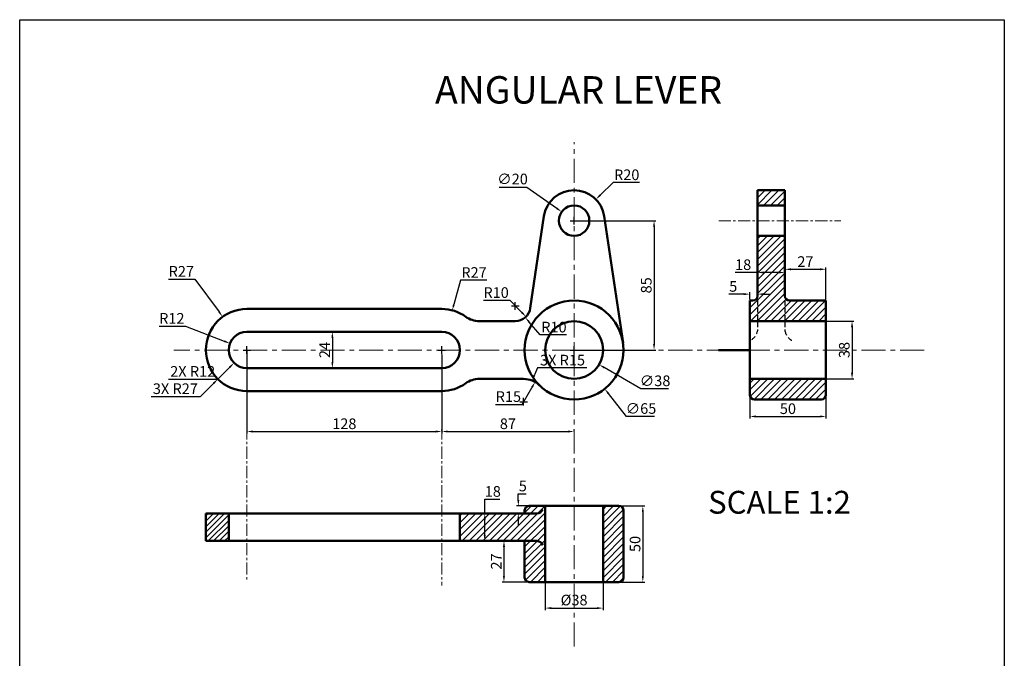
# Model space of a CAD drawing. Units: millimetres. Extents: x 161 to 808, y -21 to 750.
# Tile 2 of 2: x 161 to 808, y 330 to 750. Entities that reach past the tile are written whole.
import ezdxf

# ---------------------------------------------------------------- set-up
doc = ezdxf.new("R2010")
doc.units = ezdxf.units.MM
doc.header["$LTSCALE"] = 0.5
doc.linetypes.add('CENTER', pattern=[50.8, 31.75, -6.35, 6.35, -6.35])
doc.linetypes.add('DASHED', pattern=[19.05, 12.7, -6.35])
for name, color, linetype, lineweight in [('M-CNTR', 1, 'CENTER', 18), ('M-DIMS', 2, 'Continuous', 25), ('M-HATC', 8, 'Continuous', 18), ('M-HIDN', 6, 'DASHED', 25), ('M-OUTL', 7, 'Continuous', 50), ('M-TEXT', 3, 'Continuous', 25), ('M-TTLB', 7, 'Continuous', 25)]:
    doc.layers.add(name, color=color, linetype=linetype, lineweight=lineweight)
doc.styles.get("Standard").update_dxf_attribs({"font": 'arial.ttf'})
doc.dimstyles.new('ISO-25', dxfattribs={"dimtxt": 7, "dimasz": 4, "dimexe": 1.25, "dimexo": 0.625, "dimtad": 1, "dimtoh": 1, "dimtxsty": 'Standard', "dimcen": 2.5, "dimadec": 0, "dimazin": 0, "dimtfac": 1, "dimtofl": 0, "dimtmove": 0, "dimatfit": 3, "dimfxl": 1, "dimarcsym": 0})

# ---------------------------------------------------------------- blocks, each defined once
blk = doc.blocks.new('*D1')
at = {"layer": 'Defpoints', "color": 0, "ltscale": 0.5, "transparency": 16777216}
for p in [(294.56, 554.39), (310.51, 532.61)]:
    blk.add_point(p, dxfattribs=at)
at = {"layer": 'M-DIMS', "color": 0, "lineweight": -2, "ltscale": 0.5, "transparency": 16777216}
for p, q in [((258.99, 579.26), (276.35, 579.26)), ((276.35, 579.26), (292.2, 557.62)), ((308.01, 532.61), (313.01, 532.61)), ((310.51, 530.11), (310.51, 535.11))]:
    blk.add_line(p, q, dxfattribs=at)
at = {"layer": 'M-DIMS', "color": 0, "ltscale": 0.5, "transparency": 16777216}
blk.add_solid([(292.73, 558.01), (291.66, 557.23), (294.56, 554.39)], dxfattribs=at)
at = {"layer": 'M-DIMS', "color": 0, "ltscale": 0.5, "transparency": 16777216, "insert": (267.36, 583.4), "char_height": 7, "attachment_point": 5}
blk.add_mtext('R27', dxfattribs=at)
blk = doc.blocks.new('*D2')
at = {"layer": 'Defpoints', "color": 0, "ltscale": 0.5, "transparency": 16777216}
for p in [(299.33, 536.97), (310.51, 532.61)]:
    blk.add_point(p, dxfattribs=at)
at = {"layer": 'M-DIMS', "color": 0, "lineweight": -2, "ltscale": 0.5, "transparency": 16777216}
for p, q in [((252.81, 548.36), (270.09, 548.36)), ((270.09, 548.36), (295.6, 538.42)), ((308.01, 532.61), (313.01, 532.61)), ((310.51, 530.11), (310.51, 535.11))]:
    blk.add_line(p, q, dxfattribs=at)
at = {"layer": 'M-DIMS', "color": 0, "ltscale": 0.5, "transparency": 16777216}
blk.add_solid([(295.85, 539.04), (295.36, 537.8), (299.33, 536.97)], dxfattribs=at)
at = {"layer": 'M-DIMS', "color": 0, "ltscale": 0.5, "transparency": 16777216, "insert": (261.14, 552.5), "char_height": 7, "attachment_point": 5}
blk.add_mtext('R12', dxfattribs=at)
blk = doc.blocks.new('*D3')
at = {"layer": 'Defpoints', "color": 0, "ltscale": 0.5, "transparency": 16777216}
for p in [(486.86, 561.61), (493.9, 554.51)]:
    blk.add_point(p, dxfattribs=at)
at = {"layer": 'M-DIMS', "color": 0, "lineweight": -2, "ltscale": 0.5, "transparency": 16777216}
for p, q in [((465.9, 565.26), (483.23, 565.26)), ((483.23, 565.26), (491.08, 557.35))]:
    blk.add_line(p, q, dxfattribs=at)
at = {"layer": 'M-DIMS', "color": 0, "ltscale": 0.5, "transparency": 16777216}
blk.add_solid([(491.56, 557.82), (490.61, 556.88), (493.9, 554.51)], dxfattribs=at)
at = {"layer": 'M-DIMS', "color": 0, "ltscale": 0.5, "transparency": 16777216, "insert": (474.25, 569.46), "char_height": 7, "attachment_point": 5}
blk.add_mtext('R10', dxfattribs=at)
blk = doc.blocks.new('*D4')
at = {"layer": 'Defpoints', "color": 0, "ltscale": 0.5, "transparency": 16777216}
for p in [(445.48, 558.69), (438.51, 532.61)]:
    blk.add_point(p, dxfattribs=at)
at = {"layer": 'M-DIMS', "color": 0, "lineweight": -2, "ltscale": 0.5, "transparency": 16777216}
for p, q in [((450.77, 578.5), (446.51, 562.56)), ((468.12, 578.5), (450.77, 578.5)), ((436.01, 532.61), (441.01, 532.61)), ((438.51, 530.11), (438.51, 535.11))]:
    blk.add_line(p, q, dxfattribs=at)
at = {"layer": 'M-DIMS', "color": 0, "ltscale": 0.5, "transparency": 16777216}
blk.add_solid([(445.87, 562.73), (447.16, 562.39), (445.48, 558.69)], dxfattribs=at)
at = {"layer": 'M-DIMS', "color": 0, "ltscale": 0.5, "transparency": 16777216, "insert": (459.76, 582.64), "char_height": 7, "attachment_point": 5}
blk.add_mtext('R27', dxfattribs=at)
blk = doc.blocks.new('*D5')
at = {"layer": 'Defpoints', "color": 0, "ltscale": 0.5, "transparency": 16777216}
for p in [(539.81, 631.6), (525.51, 617.61)]:
    blk.add_point(p, dxfattribs=at)
at = {"layer": 'M-DIMS', "color": 0, "lineweight": -2, "ltscale": 0.5, "transparency": 16777216}
for p, q in [((551.11, 642.66), (542.66, 634.4)), ((568.44, 642.66), (551.11, 642.66)), ((523.01, 617.61), (528.01, 617.61)), ((525.51, 615.11), (525.51, 620.11))]:
    blk.add_line(p, q, dxfattribs=at)
at = {"layer": 'M-DIMS', "color": 0, "ltscale": 0.5, "transparency": 16777216}
blk.add_solid([(542.2, 634.87), (543.13, 633.92), (539.81, 631.6)], dxfattribs=at)
at = {"layer": 'M-DIMS', "color": 0, "ltscale": 0.5, "transparency": 16777216, "insert": (560.09, 646.86), "char_height": 7, "attachment_point": 5}
blk.add_mtext('R20', dxfattribs=at)
blk = doc.blocks.new('*D6')
at = {"layer": 'Defpoints', "color": 0, "ltscale": 0.5, "transparency": 16777216}
for p in [(509.1, 542.18), (541.92, 523.03)]:
    blk.add_point(p, dxfattribs=at)
at = {"layer": 'M-DIMS', "color": 0, "lineweight": -2, "ltscale": 0.5, "transparency": 16777216}
for p, q in [((523.01, 532.61), (528.01, 532.61)), ((525.51, 530.11), (525.51, 535.11)), ((569.29, 507.07), (545.38, 521.02)), ((587.57, 507.07), (569.29, 507.07))]:
    blk.add_line(p, q, dxfattribs=at)
at = {"layer": 'M-DIMS', "color": 0, "ltscale": 0.5, "transparency": 16777216}
blk.add_solid([(545.71, 521.59), (545.04, 520.44), (541.92, 523.03)], dxfattribs=at)
at = {"layer": 'M-DIMS', "color": 0, "ltscale": 0.5, "transparency": 16777216, "insert": (578.74, 511.46), "char_height": 7, "attachment_point": 5}
blk.add_mtext('∅38', dxfattribs=at)
blk = doc.blocks.new('*D7')
at = {"layer": 'Defpoints', "color": 0, "ltscale": 0.5, "transparency": 16777216}
for p in [(505.4, 558.14), (545.63, 507.08)]:
    blk.add_point(p, dxfattribs=at)
at = {"layer": 'M-DIMS', "color": 0, "lineweight": -2, "ltscale": 0.5, "transparency": 16777216}
for p, q in [((523.01, 532.61), (528.01, 532.61)), ((525.51, 530.11), (525.51, 535.11)), ((559.99, 488.86), (548.1, 503.94)), ((578.31, 488.86), (559.99, 488.86))]:
    blk.add_line(p, q, dxfattribs=at)
at = {"layer": 'M-DIMS', "color": 0, "ltscale": 0.5, "transparency": 16777216}
blk.add_solid([(548.63, 504.35), (547.58, 503.53), (545.63, 507.08)], dxfattribs=at)
at = {"layer": 'M-DIMS', "color": 0, "ltscale": 0.5, "transparency": 16777216, "insert": (569.46, 493.25), "char_height": 7, "attachment_point": 5}
blk.add_mtext('∅65', dxfattribs=at)
blk = doc.blocks.new('*D8')
at = {"layer": 'Defpoints', "color": 0, "ltscale": 0.5, "transparency": 16777216}
for p in [(517.37, 623.41), (533.66, 611.81)]:
    blk.add_point(p, dxfattribs=at)
at = {"layer": 'M-DIMS', "color": 0, "lineweight": -2, "ltscale": 0.5, "transparency": 16777216}
for p, q in [((476.23, 639.71), (494.48, 639.71)), ((494.48, 639.71), (514.11, 625.73)), ((523.01, 617.61), (528.01, 617.61)), ((525.51, 615.11), (525.51, 620.11))]:
    blk.add_line(p, q, dxfattribs=at)
at = {"layer": 'M-DIMS', "color": 0, "ltscale": 0.5, "transparency": 16777216}
blk.add_solid([(514.49, 626.27), (513.72, 625.19), (517.37, 623.41)], dxfattribs=at)
at = {"layer": 'M-DIMS', "color": 0, "ltscale": 0.5, "transparency": 16777216, "insert": (485.04, 644.1), "char_height": 7, "attachment_point": 5}
blk.add_mtext('∅20', dxfattribs=at)
blk = doc.blocks.new('*D9')
at = {"layer": 'Defpoints', "color": 0, "ltscale": 0.5, "transparency": 16777216}
for p in [(373.17, 544.61), (366.64, 520.61), (374.51, 520.61)]:
    blk.add_point(p, dxfattribs=at)
at = {"layer": 'M-DIMS', "color": 0, "lineweight": -2, "ltscale": 0.5, "transparency": 16777216}
for p, q in [((372.54, 544.61), (365.39, 544.61)), ((366.64, 540.61), (366.64, 524.61)), ((373.89, 520.61), (365.39, 520.61))]:
    blk.add_line(p, q, dxfattribs=at)
at = {"layer": 'M-DIMS', "color": 0, "ltscale": 0.5, "transparency": 16777216}
for points in [[(365.97, 540.61), (367.3, 540.61), (366.64, 544.61)], [(365.97, 524.61), (367.3, 524.61), (366.64, 520.61)]]:
    blk.add_solid(points, dxfattribs=at)
at = {"layer": 'M-DIMS', "color": 0, "ltscale": 0.5, "transparency": 16777216, "insert": (362.5, 532.61), "char_height": 7, "attachment_point": 5, "rotation": 90}
blk.add_mtext('24', dxfattribs=at)
blk = doc.blocks.new('*D10')
at = {"layer": 'Defpoints', "color": 0, "ltscale": 0.5, "transparency": 16777216}
for p in [(310.51, 532.61), (438.51, 530.11), (438.51, 479.03)]:
    blk.add_point(p, dxfattribs=at)
at = {"layer": 'M-DIMS', "color": 0, "lineweight": -2, "ltscale": 0.5, "transparency": 16777216}
for p, q in [((310.51, 531.98), (310.51, 477.78)), ((438.51, 529.48), (438.51, 477.78)), ((314.51, 479.03), (434.51, 479.03))]:
    blk.add_line(p, q, dxfattribs=at)
at = {"layer": 'M-DIMS', "color": 0, "ltscale": 0.5, "transparency": 16777216}
for points in [[(314.51, 479.69), (314.51, 478.36), (310.51, 479.03)], [(434.51, 479.69), (434.51, 478.36), (438.51, 479.03)]]:
    blk.add_solid(points, dxfattribs=at)
at = {"layer": 'M-DIMS', "color": 0, "ltscale": 0.5, "transparency": 16777216, "insert": (374.51, 483.22), "char_height": 7, "attachment_point": 5}
blk.add_mtext('128', dxfattribs=at)
blk = doc.blocks.new('*D11')
at = {"layer": 'Defpoints', "color": 0, "ltscale": 0.5, "transparency": 16777216}
for p in [(525.51, 617.61), (525.51, 532.61), (578.05, 532.61)]:
    blk.add_point(p, dxfattribs=at)
at = {"layer": 'M-DIMS', "color": 0, "lineweight": -2, "ltscale": 0.5, "transparency": 16777216}
for p, q in [((526.14, 617.61), (579.3, 617.61)), ((578.05, 613.61), (578.05, 536.61)), ((526.14, 532.61), (579.3, 532.61))]:
    blk.add_line(p, q, dxfattribs=at)
at = {"layer": 'M-DIMS', "color": 0, "ltscale": 0.5, "transparency": 16777216}
for points in [[(577.39, 613.61), (578.72, 613.61), (578.05, 617.61)], [(577.39, 536.61), (578.72, 536.61), (578.05, 532.61)]]:
    blk.add_solid(points, dxfattribs=at)
at = {"layer": 'M-DIMS', "color": 0, "ltscale": 0.5, "transparency": 16777216, "insert": (573.85, 575.11), "char_height": 7, "attachment_point": 5, "rotation": 90}
blk.add_mtext('85', dxfattribs=at)
blk = doc.blocks.new('*D12')
at = {"layer": 'Defpoints', "color": 0, "ltscale": 0.5, "transparency": 16777216}
for p in [(438.51, 479.03), (525.51, 479.03), (525.51, 479.03)]:
    blk.add_point(p, dxfattribs=at)
at = {"layer": 'M-DIMS', "color": 0, "lineweight": -2, "ltscale": 0.5, "transparency": 16777216}
for p, q in [((438.51, 479.65), (438.51, 480.28)), ((442.51, 479.03), (521.51, 479.03)), ((525.51, 479.65), (525.51, 480.28))]:
    blk.add_line(p, q, dxfattribs=at)
at = {"layer": 'M-DIMS', "color": 0, "ltscale": 0.5, "transparency": 16777216}
for points in [[(442.51, 479.69), (442.51, 478.36), (438.51, 479.03)], [(521.51, 479.69), (521.51, 478.36), (525.51, 479.03)]]:
    blk.add_solid(points, dxfattribs=at)
at = {"layer": 'M-DIMS', "color": 0, "ltscale": 0.5, "transparency": 16777216, "insert": (482.01, 483.22), "char_height": 7, "attachment_point": 5}
blk.add_mtext('87', dxfattribs=at)
blk = doc.blocks.new('*D13')
at = {"layer": 'Defpoints', "color": 0, "ltscale": 0.5, "transparency": 16777216}
for p in [(506.51, 380.12), (544.51, 380.12), (544.51, 362.97)]:
    blk.add_point(p, dxfattribs=at)
at = {"layer": 'M-DIMS', "color": 0, "lineweight": -2, "ltscale": 0.5, "transparency": 16777216}
for p, q in [((506.51, 379.49), (506.51, 361.72)), ((544.51, 379.49), (544.51, 361.72)), ((510.51, 362.97), (540.51, 362.97))]:
    blk.add_line(p, q, dxfattribs=at)
at = {"layer": 'M-DIMS', "color": 0, "ltscale": 0.5, "transparency": 16777216}
for points in [[(510.51, 363.64), (510.51, 362.31), (506.51, 362.97)], [(540.51, 363.64), (540.51, 362.31), (544.51, 362.97)]]:
    blk.add_solid(points, dxfattribs=at)
at = {"layer": 'M-DIMS', "color": 0, "ltscale": 0.5, "transparency": 16777216, "insert": (525.51, 367.37), "char_height": 7, "attachment_point": 5}
blk.add_mtext('%%C38', dxfattribs=at)
blk = doc.blocks.new('*D14')
at = {"layer": 'Defpoints', "color": 0, "ltscale": 0.5, "transparency": 16777216}
for p in [(496.01, 430.12), (488.86, 425.12), (496.01, 425.12)]:
    blk.add_point(p, dxfattribs=at)
at = {"layer": 'M-DIMS', "color": 0, "lineweight": -2, "ltscale": 0.5, "transparency": 16777216}
for p, q in [((488.86, 434.12), (488.86, 438.12)), ((488.86, 438.12), (494.12, 438.12)), ((495.39, 430.12), (487.61, 430.12)), ((495.39, 425.12), (487.61, 425.12)), ((488.86, 421.12), (488.86, 417.12))]:
    blk.add_line(p, q, dxfattribs=at)
at = {"layer": 'M-DIMS', "color": 0, "ltscale": 0.5, "transparency": 16777216}
for points in [[(488.19, 434.12), (489.53, 434.12), (488.86, 430.12)], [(488.19, 421.12), (489.53, 421.12), (488.86, 425.12)]]:
    blk.add_solid(points, dxfattribs=at)
at = {"layer": 'M-DIMS', "color": 0, "ltscale": 0.5, "transparency": 16777216, "insert": (491.8, 442.3), "char_height": 7, "attachment_point": 5}
blk.add_mtext('5', dxfattribs=at)
blk = doc.blocks.new('*D15')
at = {"layer": 'Defpoints', "color": 0, "ltscale": 0.5, "transparency": 16777216}
for p in [(479.65, 425.12), (466.78, 407.12), (479.65, 407.12)]:
    blk.add_point(p, dxfattribs=at)
at = {"layer": 'M-DIMS', "color": 0, "lineweight": -2, "ltscale": 0.5, "transparency": 16777216}
for p, q in [((466.78, 425.12), (466.78, 434.55)), ((466.78, 434.55), (476.79, 434.55)), ((479.03, 425.12), (465.53, 425.12)), ((466.78, 411.12), (466.78, 421.12)), ((479.03, 407.12), (465.53, 407.12))]:
    blk.add_line(p, q, dxfattribs=at)
at = {"layer": 'M-DIMS', "color": 0, "ltscale": 0.5, "transparency": 16777216}
for points in [[(466.11, 421.12), (467.45, 421.12), (466.78, 425.12)], [(466.11, 411.12), (467.45, 411.12), (466.78, 407.12)]]:
    blk.add_solid(points, dxfattribs=at)
at = {"layer": 'M-DIMS', "color": 0, "ltscale": 0.5, "transparency": 16777216, "insert": (472.1, 438.75), "char_height": 7, "attachment_point": 5}
blk.add_mtext('18', dxfattribs=at)
blk = doc.blocks.new('*D16')
at = {"layer": 'Defpoints', "color": 0, "ltscale": 0.5, "transparency": 16777216}
for p in [(691.04, 551.61), (691.04, 513.61), (708.18, 513.61)]:
    blk.add_point(p, dxfattribs=at)
at = {"layer": 'M-DIMS', "color": 0, "lineweight": -2, "ltscale": 0.5, "transparency": 16777216}
for p, q in [((691.66, 551.61), (709.43, 551.61)), ((708.18, 547.61), (708.18, 517.61)), ((691.66, 513.61), (709.43, 513.61))]:
    blk.add_line(p, q, dxfattribs=at)
at = {"layer": 'M-DIMS', "color": 0, "ltscale": 0.5, "transparency": 16777216}
for points in [[(707.52, 547.61), (708.85, 547.61), (708.18, 551.61)], [(707.52, 517.61), (708.85, 517.61), (708.18, 513.61)]]:
    blk.add_solid(points, dxfattribs=at)
at = {"layer": 'M-DIMS', "color": 0, "ltscale": 0.5, "transparency": 16777216, "insert": (703.98, 532.61), "char_height": 7, "attachment_point": 5, "rotation": 90}
blk.add_mtext('38', dxfattribs=at)
blk = doc.blocks.new('*D17')
at = {"layer": 'Defpoints', "color": 0, "ltscale": 0.5, "transparency": 16777216}
for p in [(641.04, 565.11), (646.04, 569.32), (646.04, 565.11)]:
    blk.add_point(p, dxfattribs=at)
at = {"layer": 'M-DIMS', "color": 0, "lineweight": -2, "ltscale": 0.5, "transparency": 16777216}
for p, q in [((641.04, 565.73), (641.04, 570.57)), ((646.04, 565.73), (646.04, 570.57)), ((637.04, 569.32), (627.15, 569.32)), ((650.04, 569.32), (654.04, 569.32))]:
    blk.add_line(p, q, dxfattribs=at)
at = {"layer": 'M-DIMS', "color": 0, "ltscale": 0.5, "transparency": 16777216}
for points in [[(637.04, 569.98), (637.04, 568.65), (641.04, 569.32)], [(650.04, 569.98), (650.04, 568.65), (646.04, 569.32)]]:
    blk.add_solid(points, dxfattribs=at)
at = {"layer": 'M-DIMS', "color": 0, "ltscale": 0.5, "transparency": 16777216, "insert": (630.09, 573.5), "char_height": 7, "attachment_point": 5}
blk.add_mtext('5', dxfattribs=at)
blk = doc.blocks.new('*D18')
at = {"layer": 'Defpoints', "color": 0, "ltscale": 0.5, "transparency": 16777216}
for p in [(664.04, 583.58), (646.04, 576.02), (664.04, 576.02)]:
    blk.add_point(p, dxfattribs=at)
at = {"layer": 'M-DIMS', "color": 0, "lineweight": -2, "ltscale": 0.5, "transparency": 16777216}
for p, q in [((646.04, 583.58), (631.29, 583.58)), ((646.04, 576.65), (646.04, 584.83)), ((660.04, 583.58), (650.04, 583.58)), ((664.04, 576.65), (664.04, 584.83))]:
    blk.add_line(p, q, dxfattribs=at)
at = {"layer": 'M-DIMS', "color": 0, "ltscale": 0.5, "transparency": 16777216}
for points in [[(650.04, 584.24), (650.04, 582.91), (646.04, 583.58)], [(660.04, 584.24), (660.04, 582.91), (664.04, 583.58)]]:
    blk.add_solid(points, dxfattribs=at)
at = {"layer": 'M-DIMS', "color": 0, "ltscale": 0.5, "transparency": 16777216, "insert": (636.61, 587.78), "char_height": 7, "attachment_point": 5}
blk.add_mtext('18', dxfattribs=at)
blk = doc.blocks.new('*D19')
at = {"layer": 'Defpoints', "color": 0, "ltscale": 0.5, "transparency": 16777216}
for p in [(691.04, 585.66), (664.04, 573.15), (691.04, 565.11)]:
    blk.add_point(p, dxfattribs=at)
at = {"layer": 'M-DIMS', "color": 0, "lineweight": -2, "ltscale": 0.5, "transparency": 16777216}
for p, q in [((664.04, 573.77), (664.04, 586.91)), ((668.04, 585.66), (687.04, 585.66)), ((691.04, 565.73), (691.04, 586.91))]:
    blk.add_line(p, q, dxfattribs=at)
at = {"layer": 'M-DIMS', "color": 0, "ltscale": 0.5, "transparency": 16777216}
for points in [[(668.04, 586.32), (668.04, 584.99), (664.04, 585.66)], [(687.04, 586.32), (687.04, 584.99), (691.04, 585.66)]]:
    blk.add_solid(points, dxfattribs=at)
at = {"layer": 'M-DIMS', "color": 0, "ltscale": 0.5, "transparency": 16777216, "insert": (677.54, 589.8), "char_height": 7, "attachment_point": 5}
blk.add_mtext('27', dxfattribs=at)
blk = doc.blocks.new('*D21')
at = {"layer": 'Defpoints', "color": 0, "ltscale": 0.5, "transparency": 16777216}
for p in [(479.65, 407.12), (479.42, 380.12), (501.87, 380.12)]:
    blk.add_point(p, dxfattribs=at)
at = {"layer": 'M-DIMS', "color": 0, "lineweight": -2, "ltscale": 0.5, "transparency": 16777216}
for p, q in [((479.03, 407.12), (478.17, 407.12)), ((479.42, 403.12), (479.42, 384.12)), ((501.24, 380.12), (478.17, 380.12))]:
    blk.add_line(p, q, dxfattribs=at)
at = {"layer": 'M-DIMS', "color": 0, "ltscale": 0.5, "transparency": 16777216}
for points in [[(478.75, 403.12), (480.09, 403.12), (479.42, 407.12)], [(478.75, 384.12), (480.09, 384.12), (479.42, 380.12)]]:
    blk.add_solid(points, dxfattribs=at)
at = {"layer": 'M-DIMS', "color": 0, "ltscale": 0.5, "transparency": 16777216, "insert": (475.28, 393.62), "char_height": 7, "attachment_point": 5, "rotation": 90}
blk.add_mtext('27', dxfattribs=at)
blk = doc.blocks.new('*D22')
at = {"layer": 'Defpoints', "color": 0, "ltscale": 0.5, "transparency": 16777216}
for p in [(549.73, 430.12), (549.73, 380.12), (570.69, 380.12)]:
    blk.add_point(p, dxfattribs=at)
at = {"layer": 'M-DIMS', "color": 0, "lineweight": -2, "ltscale": 0.5, "transparency": 16777216}
for p, q in [((550.35, 430.12), (571.94, 430.12)), ((570.69, 426.12), (570.69, 384.12)), ((550.35, 380.12), (571.94, 380.12))]:
    blk.add_line(p, q, dxfattribs=at)
at = {"layer": 'M-DIMS', "color": 0, "ltscale": 0.5, "transparency": 16777216}
for points in [[(570.02, 426.12), (571.36, 426.12), (570.69, 430.12)], [(570.02, 384.12), (571.36, 384.12), (570.69, 380.12)]]:
    blk.add_solid(points, dxfattribs=at)
at = {"layer": 'M-DIMS', "color": 0, "ltscale": 0.5, "transparency": 16777216, "insert": (566.49, 405.12), "char_height": 7, "attachment_point": 5, "rotation": 90}
blk.add_mtext('50', dxfattribs=at)
blk = doc.blocks.new('*D23')
at = {"layer": 'Defpoints', "color": 0, "ltscale": 0.5, "transparency": 16777216}
for p in [(641.04, 507.67), (691.04, 507.67), (691.04, 488.93)]:
    blk.add_point(p, dxfattribs=at)
at = {"layer": 'M-DIMS', "color": 0, "lineweight": -2, "ltscale": 0.5, "transparency": 16777216}
for p, q in [((641.04, 507.05), (641.04, 487.68)), ((691.04, 507.05), (691.04, 487.68)), ((645.04, 488.93), (687.04, 488.93))]:
    blk.add_line(p, q, dxfattribs=at)
at = {"layer": 'M-DIMS', "color": 0, "ltscale": 0.5, "transparency": 16777216}
for points in [[(645.04, 489.59), (645.04, 488.26), (641.04, 488.93)], [(687.04, 489.59), (687.04, 488.26), (691.04, 488.93)]]:
    blk.add_solid(points, dxfattribs=at)
at = {"layer": 'M-DIMS', "color": 0, "ltscale": 0.5, "transparency": 16777216, "insert": (666.04, 493.13), "char_height": 7, "attachment_point": 5}
blk.add_mtext('50', dxfattribs=at)
blk = doc.blocks.new('*D46')
at = {"layer": 'Defpoints', "color": 0, "ltscale": 0.5, "transparency": 16777216}
for p in [(499.89, 511.57), (492.34, 498.61)]:
    blk.add_point(p, dxfattribs=at)
at = {"layer": 'M-DIMS', "color": 0, "lineweight": -2, "ltscale": 0.5, "transparency": 16777216}
for p, q in [((491.33, 496.87), (497.88, 508.11)), ((473.92, 496.87), (491.33, 496.87))]:
    blk.add_line(p, q, dxfattribs=at)
at = {"layer": 'M-DIMS', "color": 0, "ltscale": 0.5, "transparency": 16777216}
blk.add_solid([(497.3, 508.45), (498.45, 507.78), (499.89, 511.57)], dxfattribs=at)
at = {"layer": 'M-DIMS', "color": 0, "ltscale": 0.5, "transparency": 16777216, "insert": (482.31, 501.07), "char_height": 7, "attachment_point": 5}
blk.add_mtext('R15', dxfattribs=at)
blk = doc.blocks.new('*D47')
at = {"layer": 'Defpoints', "color": 0, "ltscale": 0.5, "transparency": 16777216}
for p in [(310.51, 532.61), (291.42, 513.52)]:
    blk.add_point(p, dxfattribs=at)
at = {"layer": 'M-DIMS', "color": 0, "lineweight": -2, "ltscale": 0.5, "transparency": 16777216}
for p, q in [((308.01, 532.61), (313.01, 532.61)), ((310.51, 530.11), (310.51, 535.11)), ((279.96, 502.06), (288.59, 510.69)), ((247.58, 502.06), (279.96, 502.06))]:
    blk.add_line(p, q, dxfattribs=at)
at = {"layer": 'M-DIMS', "color": 0, "ltscale": 0.5, "transparency": 16777216}
blk.add_solid([(288.12, 511.16), (289.06, 510.22), (291.42, 513.52)], dxfattribs=at)
at = {"layer": 'M-DIMS', "color": 0, "ltscale": 0.5, "transparency": 16777216, "insert": (263.46, 506.27), "char_height": 7, "attachment_point": 5}
blk.add_mtext('3X R27', dxfattribs=at)
blk = doc.blocks.new('*D48')
at = {"layer": 'Defpoints', "color": 0, "ltscale": 0.5, "transparency": 16777216}
for p in [(310.51, 532.61), (302.03, 524.13)]:
    blk.add_point(p, dxfattribs=at)
at = {"layer": 'M-DIMS', "color": 0, "lineweight": -2, "ltscale": 0.5, "transparency": 16777216}
for p, q in [((308.01, 532.61), (313.01, 532.61)), ((310.51, 530.11), (310.51, 535.11)), ((291.39, 513.5), (299.2, 521.3)), ((258.95, 513.5), (291.39, 513.5))]:
    blk.add_line(p, q, dxfattribs=at)
at = {"layer": 'M-DIMS', "color": 0, "ltscale": 0.5, "transparency": 16777216}
blk.add_solid([(298.73, 521.77), (299.67, 520.83), (302.03, 524.13)], dxfattribs=at)
at = {"layer": 'M-DIMS', "color": 0, "ltscale": 0.5, "transparency": 16777216, "insert": (274.86, 517.64), "char_height": 7, "attachment_point": 5}
blk.add_mtext('2X R12', dxfattribs=at)
blk = doc.blocks.new('*D49')
at = {"layer": 'Defpoints', "color": 0, "ltscale": 0.5, "transparency": 16777216}
for p in [(498, 512.5), (492.34, 498.61)]:
    blk.add_point(p, dxfattribs=at)
at = {"layer": 'M-DIMS', "color": 0, "lineweight": -2, "ltscale": 0.5, "transparency": 16777216}
for p, q in [((501.39, 520.84), (499.5, 516.21)), ((533.83, 520.84), (501.39, 520.84)), ((489.84, 498.61), (494.84, 498.61)), ((492.34, 496.11), (492.34, 501.11))]:
    blk.add_line(p, q, dxfattribs=at)
at = {"layer": 'M-DIMS', "color": 0, "ltscale": 0.5, "transparency": 16777216}
blk.add_solid([(498.89, 516.46), (500.12, 515.96), (498, 512.5)], dxfattribs=at)
at = {"layer": 'M-DIMS', "color": 0, "ltscale": 0.5, "transparency": 16777216, "insert": (517.92, 525.04), "char_height": 7, "attachment_point": 5}
blk.add_mtext('3X R15', dxfattribs=at)
blk = doc.blocks.new('*D50')
at = {"layer": 'Defpoints', "color": 0, "ltscale": 0.5, "transparency": 16777216}
for p in [(486.86, 561.61), (493.39, 554.04)]:
    blk.add_point(p, dxfattribs=at)
at = {"layer": 'M-DIMS', "color": 0, "lineweight": -2, "ltscale": 0.5, "transparency": 16777216}
for p, q in [((486.86, 559.11), (486.86, 564.11)), ((484.36, 561.61), (489.36, 561.61)), ((503.28, 542.56), (496, 551.01)), ((520.61, 542.56), (503.28, 542.56))]:
    blk.add_line(p, q, dxfattribs=at)
at = {"layer": 'M-DIMS', "color": 0, "ltscale": 0.5, "transparency": 16777216}
blk.add_solid([(496.5, 551.44), (495.49, 550.57), (493.39, 554.04)], dxfattribs=at)
at = {"layer": 'M-DIMS', "color": 0, "ltscale": 0.5, "transparency": 16777216, "insert": (512.26, 546.76), "char_height": 7, "attachment_point": 5}
blk.add_mtext('R10', dxfattribs=at)

msp = doc.modelspace()

# ---------------------------------------------------------------- hatches: boundary and pattern name
at = {"layer": 'M-HATC', "ltscale": 0.5}
h = msp.add_hatch(dxfattribs=at)
h.set_pattern_fill('ANSI31', color=256)
h.paths.add_polyline_path([(691.039, 513.61), (641.039, 513.61), (641.039, 503.11, 0.4142136), (644.039, 500.11), (688.039, 500.11, 0.4142136), (691.039, 503.11)])
h.paths.add_polyline_path([(691.039, 565.11), (667.039, 565.11, -0.4142136), (664.039, 568.11), (664.039, 607.61), (646.039, 607.61), (646.039, 568.11, -0.4142136), (643.039, 565.11), (641.039, 565.11), (641.039, 551.61), (691.039, 551.61)])
h.paths.add_polyline_path([(664.039, 637.61), (646.039, 637.61), (646.039, 627.61), (664.039, 627.61)])
h = msp.add_hatch(dxfattribs=at)
h.set_pattern_fill('ANSI31', color=256)
h.paths.add_polyline_path([(506.512, 430.119), (496.012, 430.119, 0.4142136), (493.012, 427.119), (493.012, 425.119), (450.512, 425.119), (450.512, 407.119), (493.012, 407.119), (493.012, 383.119, 0.4142136), (496.012, 380.119), (506.512, 380.119)])
h.paths.add_polyline_path([(558.012, 427.119, 0.4142136), (555.012, 430.119), (544.512, 430.119), (544.512, 380.119), (555.012, 380.119, 0.4142136), (558.012, 383.119)])
h = msp.add_hatch(dxfattribs=at)
h.set_pattern_fill('ANSI31', color=256, scale=0.8)
h.paths.add_polyline_path([(298.512, 425.119), (283.512, 425.119), (283.512, 407.119), (298.512, 407.119)])

# ---------------------------------------------------------------- linework, layer by layer
at = {"layer": 'M-CNTR'}
for p, q in [((525.512, 337.68), (525.512, 669.148)), ((755.66, 532.61), (262.525, 532.61))]:
    msp.add_line(p, q, dxfattribs=at)
at = {"layer": 'M-CNTR', "ltscale": 0.5}
for p, q in [((620.545, 617.61), (700.879, 617.61)), ((310.512, 532.61), (310.512, 381.519)), ((438.512, 532.61), (438.512, 377.901))]:
    msp.add_line(p, q, dxfattribs=at)
at = {"layer": 'M-HIDN', "ltscale": 0.5}
for p, q in [((646.039, 565.11), (646.039, 545.233)), ((664.039, 565.11), (664.039, 545.233))]:
    msp.add_line(p, q, dxfattribs=at)
for centre, start, end in [((637.145, 546.932), 305.120535, 349.187678), ((672.933, 546.932), 190.812322, 250.812322)]:
    msp.add_arc(centre, 9.055, start, end, dxfattribs=at)
at = {"layer": 'M-OUTL', "ltscale": 0.5}
for p, q in [((646.039, 568.11), (646.039, 637.61)), ((646.039, 637.61), (664.039, 637.61)), ((664.039, 637.61), (664.039, 568.11)), ((646.039, 627.61), (664.039, 627.61)), ((646.039, 607.61), (664.039, 607.61)), ((641.039, 565.11), (641.039, 503.11)), ((643.039, 565.11), (641.039, 565.11)), ((691.039, 565.11), (667.039, 565.11)), ((691.039, 503.11), (691.039, 565.11)), ((691.039, 551.61), (641.039, 551.61)), ((641.039, 532.61), (620.31, 532.61)), ((691.039, 513.61), (641.039, 513.61)), ((644.039, 500.11), (688.039, 500.11)), ((493.012, 425.119), (493.012, 427.119)), ((496.012, 430.119), (555.012, 430.119)), ((506.512, 380.119), (506.512, 430.119)), ((544.512, 380.119), (544.512, 430.119)), ((558.012, 427.119), (558.012, 383.119)), ((501.084, 425.119), (283.512, 425.119)), ((283.512, 425.119), (283.512, 407.119)), ((298.512, 425.119), (298.512, 407.119)), ((450.512, 425.119), (450.512, 407.119)), ((283.512, 407.119), (501.084, 407.119)), ((493.012, 383.119), (493.012, 407.119)), ((555.012, 380.119), (496.012, 380.119))]:
    msp.add_line(p, q, dxfattribs=at)
at = {"layer": 'M-OUTL'}
for p, q in [((505.729, 620.551), (496.747, 560.139)), ((545.294, 620.551), (557.658, 537.389)), ((310.512, 559.61), (438.512, 559.61)), ((486.856, 551.61), (463.169, 551.61)), ((310.512, 544.61), (438.512, 544.61)), ((310.512, 520.61), (438.512, 520.61)), ((492.342, 513.61), (463.169, 513.61)), ((310.512, 505.61), (438.512, 505.61))]:
    msp.add_line(p, q, dxfattribs=at)
for centre, radius in [((525.512, 617.61), 10), ((525.512, 532.61), 32.5), ((525.512, 532.61), 19)]:
    msp.add_circle(centre, radius, dxfattribs=at)
for centre, radius, start, end in [((525.512, 617.61), 20, 8.456519, 171.543481), ((310.512, 532.61), 27, 90, 270), ((438.512, 532.61), 27, 54.049432, 90), ((486.856, 561.61), 10, 270, 351.543481), ((463.169, 566.61), 15, 234.049432, 270), ((310.512, 532.61), 12, 90, 270), ((438.512, 532.61), 12, 270, 90), ((463.169, 498.61), 15, 90, 125.950568), ((492.342, 498.61), 15, 45.707937, 90), ((438.512, 532.61), 27, 270, 305.950568)]:
    msp.add_arc(centre, radius, start, end, dxfattribs=at)
at = {"layer": 'M-OUTL', "ltscale": 0.5}
for centre, radius, start, end in [((643.039, 568.11), 3, 270, 0), ((667.039, 568.11), 3, 180, 270), ((644.039, 503.11), 3, 180, 270), ((688.039, 503.11), 3, 270, 0), ((496.012, 427.119), 3, 90, 180), ((500.604, 429.823), 4.728, 275.819065, 335.819065), ((555.012, 427.119), 3, 0, 90), ((500.604, 402.415), 4.728, 24.180935, 84.180935), ((496.012, 383.119), 3, 180, 270), ((555.012, 383.119), 3, 270, 0)]:
    msp.add_arc(centre, radius, start, end, dxfattribs=at)
at = {"layer": 'M-TTLB', "ltscale": 0.5}
msp.add_lwpolyline([(161.16, 749.71), (808.244, 749.71), (808.244, -21.293), (161.16, -21.293)], close=True, dxfattribs=at)

# ---------------------------------------------------------------- texts
at = {"layer": 'M-TEXT', "ltscale": 0.5, "attachment_point": 1}
for s, width, insert, char_height in [('ANGULAR LEVER', 235.42722, (434.132, 712.597), 18), ('SCALE 1:2', 111.67008, (613.577, 440.034), 15)]:
    msp.add_mtext_dynamic_manual_height_columns(s, width=width, gutter_width=12.5, heights=[0], dxfattribs=dict(at, insert=insert, char_height=char_height))

# ---------------------------------------------------------------- dimensions: what is measured, and where the dimension line sits
at = {"layer": 'M-DIMS', "ltscale": 0.5}
for p1, p2, picture, middle in [((533.658, 611.81), (517.365, 623.409), '*D8', (485.041, 639.706)), ((505.396, 558.136), (545.628, 507.083), '*D7', (569.464, 488.857)), ((509.101, 542.185), (541.923, 523.034), '*D6', (578.743, 507.067))]:
    dim = msp.add_diameter_dim_2p(p1=p1, p2=p2, dimstyle='ISO-25', override={"dimclrd": 0, "dimclre": 0, "dimclrt": 0}, dxfattribs=at)
    dim.commit()
    dim.dimension.update_dxf_attribs({"geometry": picture, "text_midpoint": middle, "dimtype": 163})
for center, mpoint, picture, middle in [((525.512, 617.61), (539.806, 631.598), '*D5', (560.085, 642.661)), ((310.512, 532.61), (294.559, 554.393), '*D1', (267.357, 579.264)), ((438.512, 532.61), (445.481, 558.695), '*D4', (459.759, 578.497)), ((486.856, 561.61), (493.902, 554.514), '*D3', (474.253, 565.263)), ((310.512, 532.61), (299.331, 536.966), '*D2', (261.137, 548.36)), ((492.342, 498.61), (499.891, 511.571), '*D46', (482.313, 496.869))]:
    dim = msp.add_radius_dim(center=center, mpoint=mpoint, dimstyle='ISO-25', override={"dimclrd": 0, "dimclre": 0, "dimclrt": 0}, dxfattribs=at)
    dim.commit()
    dim.dimension.update_dxf_attribs({"geometry": picture, "text_midpoint": middle, "dimtype": 164})
for base, p1, p2, angle, picture, middle in [((578.053, 532.61), (525.512, 617.61), (525.512, 532.61), 90, '*D11', (573.854, 575.11)), ((691.039, 585.657), (664.039, 573.149), (691.039, 565.11), 180, '*D19', (677.539, 589.796)), ((708.184, 513.61), (691.039, 551.61), (691.039, 513.61), 270, '*D16', (703.983, 532.61)), ((366.637, 520.61), (373.17, 544.61), (374.512, 520.61), 90, '*D9', (362.498, 532.61)), ((570.69, 380.119), (549.729, 430.119), (549.729, 380.119), 90, '*D22', (566.491, 405.119)), ((479.419, 380.119), (479.652, 407.119), (501.865, 380.119), 90, '*D21', (475.28, 393.619))]:
    dim = msp.add_linear_dim(base=base, p1=p1, p2=p2, angle=angle, dimstyle='ISO-25', override={"dimclrd": 0, "dimclre": 0, "dimclrt": 0}, dxfattribs=at)
    dim.commit()
    dim.dimension.update_dxf_attribs({"geometry": picture, "text_midpoint": middle})
for base, p1, p2, angle, picture, middle in [((664.039, 583.577), (646.039, 576.022), (664.039, 576.022), 180, '*D18', (636.611, 583.577)), ((646.039, 569.317), (641.039, 565.11), (646.039, 565.11), 180, '*D17', (630.093, 569.317)), ((488.859, 425.119), (496.012, 430.119), (496.012, 425.119), 90, '*D14', (491.804, 438.119)), ((466.781, 407.119), (479.652, 425.119), (479.652, 407.119), 90, '*D15', (472.097, 434.547))]:
    dim = msp.add_linear_dim(base=base, p1=p1, p2=p2, angle=angle, dimstyle='ISO-25', override={"dimclrd": 0, "dimclre": 0, "dimclrt": 0}, dxfattribs=at)
    dim.commit()
    dim.dimension.update_dxf_attribs({"geometry": picture, "text_midpoint": middle, "dimtype": 160})
dim = msp.add_radius_dim(center=(486.856, 561.61), mpoint=(493.387, 554.036), dimstyle='ISO-25', override={"dimdec": 0, "dimlfac": 1, "dimrnd": 0, "dimzin": 0, "dimdsep": 46, "dimlunit": 2}, dxfattribs=at)
dim.commit()
dim.dimension.update_dxf_attribs({"geometry": '*D50', "text_midpoint": (512.255, 546.764)})
for center, mpoint, picture, middle in [((310.512, 532.61), (291.419, 513.519), '*D47', (263.457, 502.064)), ((492.342, 498.61), (497.996, 512.503), '*D49', (517.921, 520.839))]:
    dim = msp.add_radius_dim(center=center, mpoint=mpoint, text='3X <>', dimstyle='ISO-25', override={"dimdec": 0, "dimlfac": 1, "dimrnd": 0, "dimzin": 0, "dimdsep": 46, "dimlunit": 2}, dxfattribs=at)
    dim.commit()
    dim.dimension.update_dxf_attribs({"geometry": picture, "text_midpoint": middle, "dimtype": 164})
dim = msp.add_radius_dim(center=(310.512, 532.61), mpoint=(302.025, 524.125), text='2X <>', dimstyle='ISO-25', override={"dimdec": 0, "dimlfac": 1, "dimrnd": 0, "dimzin": 0, "dimdsep": 46, "dimlunit": 2}, dxfattribs=at)
dim.commit()
dim.dimension.update_dxf_attribs({"geometry": '*D48', "text_midpoint": (274.861, 517.638)})
for base, p1, p2, picture, middle in [((438.512, 479.026), (310.512, 532.61), (438.512, 530.11), '*D10', (374.512, 483.225)), ((691.039, 488.927), (641.039, 507.673), (691.039, 507.673), '*D23', (666.039, 493.126)), ((525.512, 479.026), (438.512, 479.026), (525.512, 479.026), '*D12', (482.012, 483.225))]:
    dim = msp.add_linear_dim(base=base, p1=p1, p2=p2, dimstyle='ISO-25', override={"dimclrd": 0, "dimclre": 0, "dimclrt": 0}, dxfattribs=at)
    dim.commit()
    dim.dimension.update_dxf_attribs({"geometry": picture, "text_midpoint": middle})
dim = msp.add_linear_dim(base=(544.512, 362.974), p1=(506.512, 380.119), p2=(544.512, 380.119), text='%%C<>', dimstyle='ISO-25', override={"dimclrd": 0, "dimclre": 0, "dimclrt": 0}, dxfattribs=at)
dim.commit()
dim.dimension.update_dxf_attribs({"geometry": '*D13', "text_midpoint": (525.512, 367.368)})

doc.saveas('drawing.dxf')
